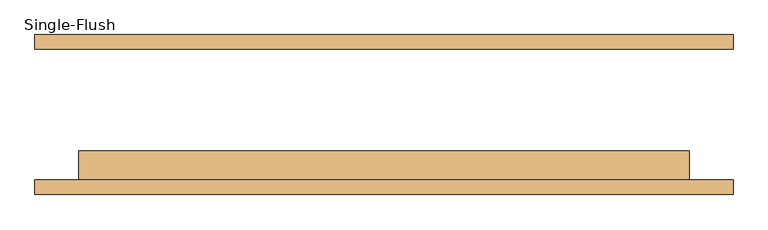
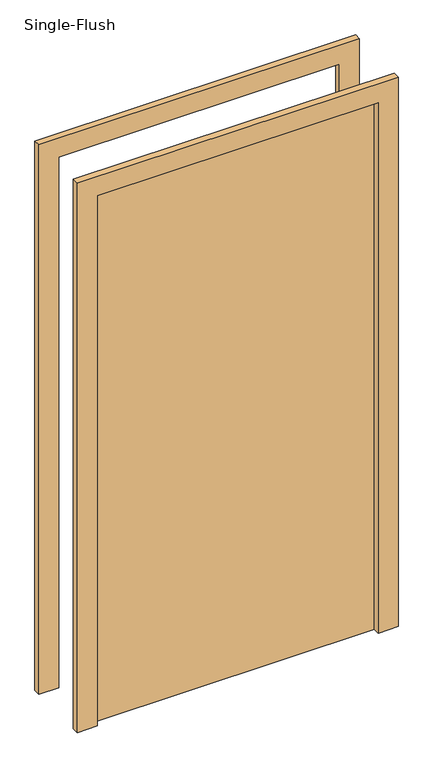
"""IFC4 building model written with IfcOpenShell, lengths in millimetres: door geometry, Single-Flush."""

from ifc_helpers import new_model, si_unit, frame, origin, origin_with_axes, place, context, project, spatial, polyline, outline, extrude, source, transform, mapped, element, save


def single_flush_0848dd25(model_context):
    return source(origin(), model_context, "Body", "SweptSolid", [
        extrude(outline(polyline([(2209.8, -609.6), (0.0, -609.6), (0.0, -533.4), (2133.6, -533.4), (2133.6, 533.4), (0.0, 533.4), (0.0, 609.6), (2209.8, 609.6), (2209.8, -609.6)])), frame((0.0, -139.7, 0.0), z_axis=(0.0, 1.0, 0.0), x_axis=(0.0, 0.0, 1.0)), (0.0, 0.0, 1.0), 25.4),
        extrude(outline(polyline([(2209.8, 609.6), (2209.8, -609.6), (0.0, -609.6), (0.0, -533.4), (2133.6, -533.4), (2133.6, 533.4), (0.0, 533.4), (0.0, 609.6), (2209.8, 609.6)])), frame((0.0, 114.3, 0.0), z_axis=(0.0, 1.0, 0.0), x_axis=(0.0, 0.0, 1.0)), (0.0, 0.0, 1.0), 25.4),
        extrude(outline(polyline([(533.4, -63.5), (533.4, -114.3), (-533.4, -114.3), (-533.4, -63.5), (533.4, -63.5)])), origin_with_axes(), (0.0, 0.0, 1.0), 2133.6),
    ])


if __name__ == "__main__":
    model = new_model("IFC4")
    model_context = context("Model", 3, world=origin())
    ifc_project = project(units=[si_unit("LENGTHUNIT", "METRE", prefix="MILLI")], contexts=[model_context])
    site = spatial("IfcSite", under=ifc_project)
    building = spatial("IfcBuilding", under=site)
    placement = place(None, origin())
    single_flush_shape = single_flush_0848dd25(model_context)
    element("IfcDoor", 1, ObjectType="Single-Flush", at=placement, inside=building, context=model_context, shape_type="MappedRepresentation", body=[
        mapped(single_flush_shape, transform((0.0, 0.0, 0.0), x_axis=(1.0, 0.0, 0.0), y_axis=(0.0, 1.0, 0.0), z_axis=(0.0, 0.0, 1.0))),
    ])
    save(model, "model.ifc")

# Revit data of these elements
# Type "Single-Flush"
#   Type Mark = "8"
#   Construction Type Id = "MDOOR"
#   Assembly Code = "C1020"
#   Analytic Construction = "Metal"
#   Thickness = 0' - 2"
#   Heat Transfer Coefficient (U) = 0.651978 BTU/(h·ft²·°F)
#   Height = 7' - 0"
#   Trim Projection Ext = 0' - 1"
#   Trim Projection Int = 0' - 1"
#   Trim Width = 0' - 3"
#   Width = 3' - 6"
#   Define Thermal Properties by = 1
#   Door Material = Door - Panel
#   Frame Material = Door - Frame
#   Visual Light Transmittance = 0
#   Solar Heat Gain Coefficient = 0
#   Function = (empty or 0)
#   Wall Closure = (empty or 0)
# Element 1 (IfcDoor, "Single-Flush")
#   Materials on its faces: "Door - Frame", "Door - Panel"
# Materials
#   "Door - Panel": class "Wood", colour RGB 210 159 95, transparency 0, Cost = 0
#   "Door - Frame": colour RGB 118 70 51, transparency 0, Cost = 0
